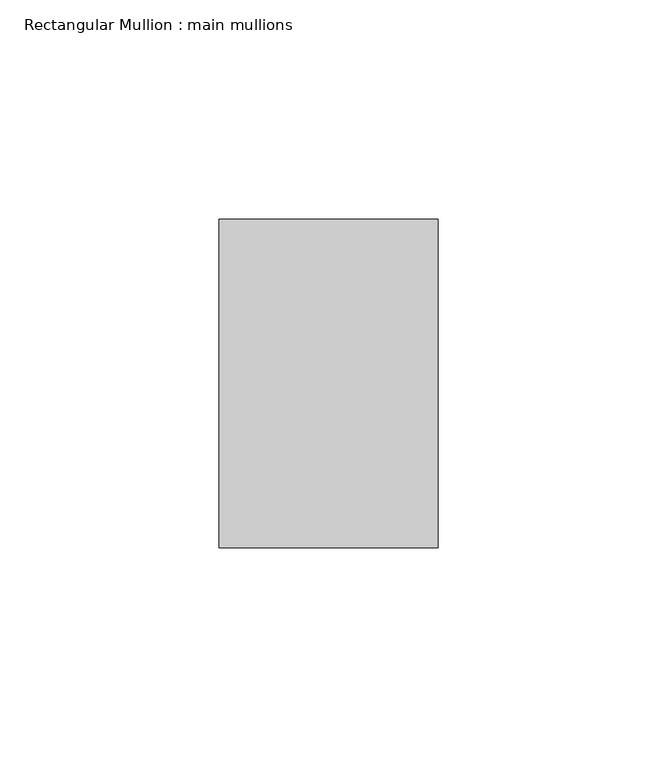
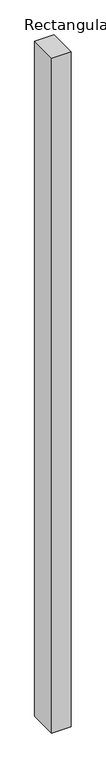
"""IFC4 building model written with IfcOpenShell, lengths in millimetres: member geometry, Rectangular Mullion : main mullions."""

from ifc_helpers import new_model, si_unit, frame, origin, place, context, project, spatial, polyline, outline, extrude, source, transform, mapped, element, save


def rectangular_mullion_main_mullions_32a4afb2(model_context):
    return source(origin(), model_context, "Body", "SweptSolid", [
        extrude(outline(polyline([(0.0, 37.5), (0.0, -37.5), (-50.0, -37.5), (-50.0, 37.5), (0.0, 37.5)])), frame((0.0, 0.0, -1825.0), z_axis=(0.0, 0.0, 1.0), x_axis=(1.0, 0.0, 0.0)), (0.0, 0.0, 1.0), 1825.0),
    ])


if __name__ == "__main__":
    model = new_model("IFC4")
    model_context = context("Model", 3, world=origin())
    ifc_project = project(units=[si_unit("LENGTHUNIT", "METRE", prefix="MILLI")], contexts=[model_context])
    site = spatial("IfcSite", under=ifc_project)
    building = spatial("IfcBuilding", under=site)
    placement = place(None, origin())
    rectangular_mullion_main_mullions_shape = rectangular_mullion_main_mullions_32a4afb2(model_context)
    element("IfcMember", 1, ObjectType="Rectangular Mullion : main mullions", at=placement, inside=building, context=model_context, shape_type="MappedRepresentation", body=[
        mapped(rectangular_mullion_main_mullions_shape, transform((0.0, 0.0, 0.0), x_axis=(1.0, 0.0, 0.0), y_axis=(0.0, 1.0, 0.0), z_axis=(0.0, 0.0, 1.0))),
    ])
    save(model, "model.ifc")

# Revit data of these elements
# Type "Rectangular Mullion : main mullions"
#   built-in parameter 1007304 = 0.246063 (stored number, unit not read)
#   built-in parameter 1007301 = 0.082021 (stored number, unit not read)
#   built-in parameter 1007300 = 0.082021 (stored number, unit not read)
# Element 1 (IfcMember, "Rectangular Mullion : main mullions")
#   Materials on its faces: "Aluminum"
# Materials
#   "Aluminum": class "Metal", colour RGB 136 136 136, transparency 0, Description = "Aluminum 6061", Cost = 0
